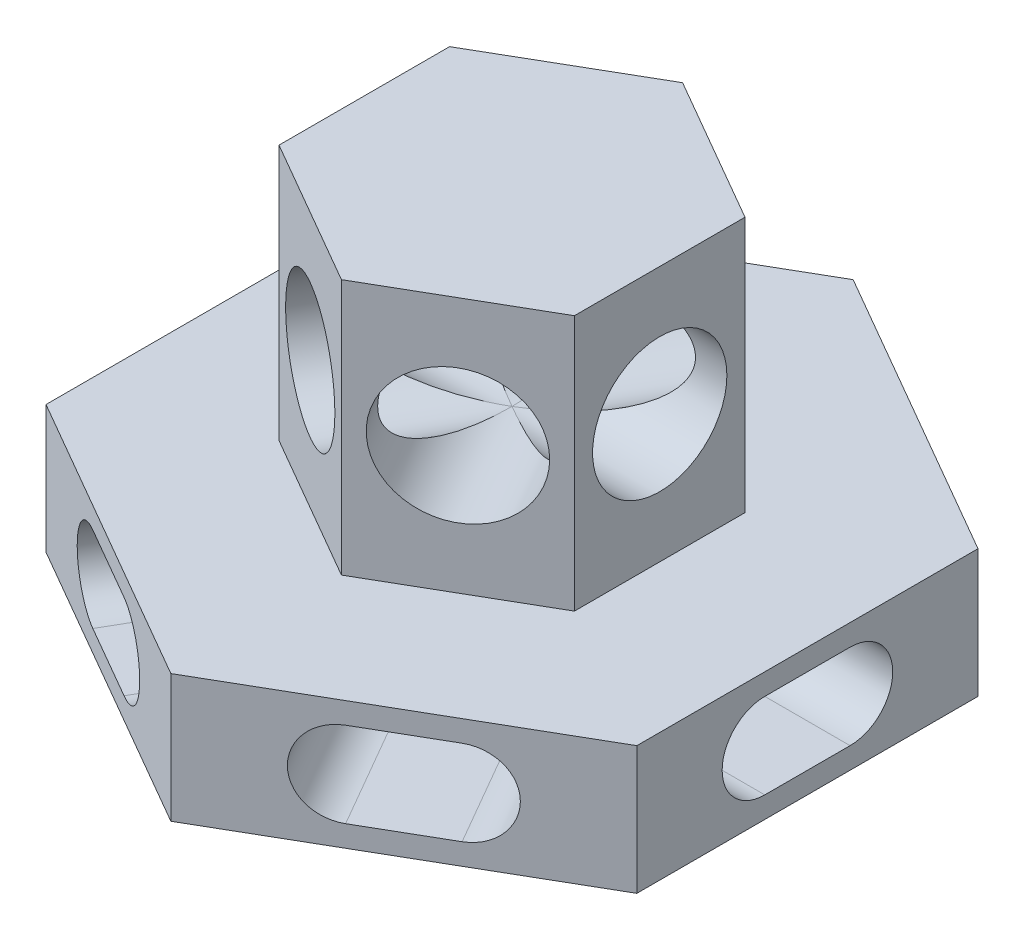
ISO-10303-21;
HEADER;
FILE_DESCRIPTION(('STEP AP214'),'2;1');
FILE_NAME('part.step','',(''),(''),'','','');
FILE_SCHEMA(('AUTOMOTIVE_DESIGN { 1 0 10303 214 1 1 1 1 }'));
ENDSEC;
DATA;
#1=APPLICATION_CONTEXT('core data for automotive mechanical design processes');
#2=APPLICATION_PROTOCOL_DEFINITION('international standard','automotive_design',2000,#1);
#3=PRODUCT_CONTEXT('',#1,'mechanical');
#4=PRODUCT('Part','Part','',(#3));
#5=PRODUCT_RELATED_PRODUCT_CATEGORY('part','',(#4));
#6=PRODUCT_DEFINITION_FORMATION('','',#4);
#7=PRODUCT_DEFINITION_CONTEXT('part definition',#1,'design');
#8=PRODUCT_DEFINITION('design','',#6,#7);
#9=PRODUCT_DEFINITION_SHAPE('','',#8);
#10=(LENGTH_UNIT() NAMED_UNIT(*) SI_UNIT(.MILLI.,.METRE.));
#11=(NAMED_UNIT(*) PLANE_ANGLE_UNIT() SI_UNIT($,.RADIAN.));
#12=(NAMED_UNIT(*) SI_UNIT($,.STERADIAN.) SOLID_ANGLE_UNIT());
#13=UNCERTAINTY_MEASURE_WITH_UNIT(LENGTH_MEASURE(1.E-05),#10,'distance_accuracy_value','');
#14=(GEOMETRIC_REPRESENTATION_CONTEXT(3) GLOBAL_UNCERTAINTY_ASSIGNED_CONTEXT((#13)) GLOBAL_UNIT_ASSIGNED_CONTEXT((#10,
#11,#12)) REPRESENTATION_CONTEXT('',''));
#15=CARTESIAN_POINT('',(0.,0.,0.));
#16=DIRECTION('',(0.,0.,1.));
#17=DIRECTION('',(1.,0.,0.));
#18=AXIS2_PLACEMENT_3D('',#15,#16,#17);
#19=CARTESIAN_POINT('',(-69.2820323027551,45.,0.));
#20=DIRECTION('',(1.,0.,0.));
#21=DIRECTION('',(0.,0.,-1.));
#22=AXIS2_PLACEMENT_3D('',#19,#20,#21);
#23=CYLINDRICAL_SURFACE('',#22,15.75);
#24=CARTESIAN_POINT('',(34.6410161513775,45.,0.));
#25=DIRECTION('',(1.,0.,0.));
#26=DIRECTION('',(0.,0.,-1.));
#27=AXIS2_PLACEMENT_3D('',#24,#25,#26);
#28=CIRCLE('',#27,15.75);
#29=CARTESIAN_POINT('',(34.6410161513775,45.,-15.75));
#30=VERTEX_POINT('',#29);
#31=EDGE_CURVE('E278',#30,#30,#28,.T.);
#32=ORIENTED_EDGE('',*,*,#31,.T.);
#33=EDGE_LOOP('',(#32));
#34=FACE_BOUND('',#33,.T.);
#35=CARTESIAN_POINT('',(0.,45.,0.));
#36=DIRECTION('',(0.5,0.,0.866025403784439));
#37=DIRECTION('',(0.866025403784439,0.,-0.5));
#38=AXIS2_PLACEMENT_3D('',#35,#36,#37);
#39=ELLIPSE('',#38,31.5,15.75);
#40=CARTESIAN_POINT('',(0.,60.75,0.));
#41=VERTEX_POINT('',#40);
#42=CARTESIAN_POINT('',(0.,29.25,0.));
#43=VERTEX_POINT('',#42);
#44=EDGE_CURVE('E262',#41,#43,#39,.F.);
#45=ORIENTED_EDGE('',*,*,#44,.T.);
#46=CARTESIAN_POINT('',(0.,45.,0.));
#47=DIRECTION('',(0.5,0.,-0.866025403784439));
#48=DIRECTION('',(0.866025403784439,0.,0.5));
#49=AXIS2_PLACEMENT_3D('',#46,#47,#48);
#50=ELLIPSE('',#49,31.5,15.75);
#51=EDGE_CURVE('E260',#43,#41,#50,.F.);
#52=ORIENTED_EDGE('',*,*,#51,.T.);
#53=EDGE_LOOP('',(#45,#52));
#54=FACE_BOUND('',#53,.T.);
#55=ADVANCED_FACE('F41',(#34,#54),#23,.F.);
#56=CARTESIAN_POINT('',(69.2820323027551,0.,-9.99999999999999));
#57=DIRECTION('',(-1.,0.,0.));
#58=DIRECTION('',(0.,0.,1.));
#59=AXIS2_PLACEMENT_3D('',#56,#57,#58);
#60=CYLINDRICAL_SURFACE('',#59,10.);
#61=DIRECTION('',(-1.,0.,0.));
#62=VECTOR('',#61,1.);
#63=CARTESIAN_POINT('',(69.2820323027551,10.,-9.99999999999999));
#64=LINE('',#63,#62);
#65=CARTESIAN_POINT('',(69.2820323027551,10.,-9.99999999999999));
#66=VERTEX_POINT('',#65);
#67=CARTESIAN_POINT('',(17.3205080756888,10.,-9.99999999999998));
#68=VERTEX_POINT('',#67);
#69=EDGE_CURVE('E438',#66,#68,#64,.T.);
#70=ORIENTED_EDGE('',*,*,#69,.T.);
#71=CARTESIAN_POINT('',(17.3205080756888,0.,-9.99999999999999));
#72=DIRECTION('',(-0.5,0.,-0.866025403784439));
#73=DIRECTION('',(-0.866025403784439,0.,0.5));
#74=AXIS2_PLACEMENT_3D('',#71,#72,#73);
#75=ELLIPSE('',#74,20.,10.);
#76=CARTESIAN_POINT('',(17.3205080756888,-10.,-9.99999999999998));
#77=VERTEX_POINT('',#76);
#78=EDGE_CURVE('E405',#68,#77,#75,.T.);
#79=ORIENTED_EDGE('',*,*,#78,.T.);
#80=DIRECTION('',(-1.,0.,0.));
#81=VECTOR('',#80,1.);
#82=CARTESIAN_POINT('',(69.2820323027551,-10.,-9.99999999999999));
#83=LINE('',#82,#81);
#84=CARTESIAN_POINT('',(69.2820323027551,-10.,-9.99999999999999));
#85=VERTEX_POINT('',#84);
#86=EDGE_CURVE('E455',#85,#77,#83,.T.);
#87=ORIENTED_EDGE('',*,*,#86,.F.);
#88=CARTESIAN_POINT('',(69.2820323027551,0.,-9.99999999999999));
#89=DIRECTION('',(-1.,0.,0.));
#90=DIRECTION('',(0.,0.,1.));
#91=AXIS2_PLACEMENT_3D('',#88,#89,#90);
#92=CIRCLE('',#91,10.);
#93=EDGE_CURVE('E414',#66,#85,#92,.T.);
#94=ORIENTED_EDGE('',*,*,#93,.F.);
#95=EDGE_LOOP('',(#70,#79,#87,#94));
#96=FACE_BOUND('',#95,.T.);
#97=ADVANCED_FACE('F525',(#96),#60,.F.);
#98=CARTESIAN_POINT('',(69.2820323027551,0.,10.));
#99=DIRECTION('',(-1.,0.,0.));
#100=DIRECTION('',(0.,0.,1.));
#101=AXIS2_PLACEMENT_3D('',#98,#99,#100);
#102=CYLINDRICAL_SURFACE('',#101,10.);
#103=DIRECTION('',(-1.,0.,0.));
#104=VECTOR('',#103,1.);
#105=CARTESIAN_POINT('',(69.2820323027551,-10.,10.));
#106=LINE('',#105,#104);
#107=CARTESIAN_POINT('',(69.2820323027551,-10.,10.));
#108=VERTEX_POINT('',#107);
#109=CARTESIAN_POINT('',(17.3205080756888,-10.,9.99999999999999));
#110=VERTEX_POINT('',#109);
#111=EDGE_CURVE('E450',#108,#110,#106,.T.);
#112=ORIENTED_EDGE('',*,*,#111,.T.);
#113=CARTESIAN_POINT('',(17.3205080756888,0.,10.));
#114=DIRECTION('',(-0.5,0.,0.866025403784439));
#115=DIRECTION('',(-0.866025403784439,0.,-0.5));
#116=AXIS2_PLACEMENT_3D('',#113,#114,#115);
#117=ELLIPSE('',#116,20.,10.);
#118=CARTESIAN_POINT('',(17.3205080756888,10.,9.99999999999999));
#119=VERTEX_POINT('',#118);
#120=EDGE_CURVE('E361',#110,#119,#117,.T.);
#121=ORIENTED_EDGE('',*,*,#120,.T.);
#122=DIRECTION('',(-1.,0.,0.));
#123=VECTOR('',#122,1.);
#124=CARTESIAN_POINT('',(69.2820323027551,10.,10.));
#125=LINE('',#124,#123);
#126=CARTESIAN_POINT('',(69.2820323027551,10.,10.));
#127=VERTEX_POINT('',#126);
#128=EDGE_CURVE('E441',#127,#119,#125,.T.);
#129=ORIENTED_EDGE('',*,*,#128,.F.);
#130=CARTESIAN_POINT('',(69.2820323027551,0.,10.));
#131=DIRECTION('',(-1.,0.,0.));
#132=DIRECTION('',(0.,0.,1.));
#133=AXIS2_PLACEMENT_3D('',#130,#131,#132);
#134=CIRCLE('',#133,10.);
#135=EDGE_CURVE('E425',#108,#127,#134,.T.);
#136=ORIENTED_EDGE('',*,*,#135,.F.);
#137=EDGE_LOOP('',(#112,#121,#129,#136));
#138=FACE_BOUND('',#137,.T.);
#139=ADVANCED_FACE('F530',(#138),#102,.F.);
#140=CARTESIAN_POINT('',(0.,15.,80.));
#141=DIRECTION('',(-0.499999999999999,0.,-0.866025403784439));
#142=DIRECTION('',(-0.866025403784439,0.,0.5));
#143=AXIS2_PLACEMENT_3D('',#140,#141,#142);
#144=PLANE('',#143);
#145=DIRECTION('',(0.866025403784439,0.,-0.5));
#146=VECTOR('',#145,1.);
#147=CARTESIAN_POINT('',(0.,10.,80.));
#148=LINE('',#147,#146);
#149=CARTESIAN_POINT('',(25.9807621135331,10.,65.));
#150=VERTEX_POINT('',#149);
#151=CARTESIAN_POINT('',(43.3012701892219,10.,55.));
#152=VERTEX_POINT('',#151);
#153=EDGE_CURVE('E360',#150,#152,#148,.T.);
#154=ORIENTED_EDGE('',*,*,#153,.T.);
#155=CARTESIAN_POINT('',(43.3012701892219,0.,55.));
#156=DIRECTION('',(-0.499999999999999,0.,-0.866025403784439));
#157=DIRECTION('',(-0.866025403784439,0.,0.5));
#158=AXIS2_PLACEMENT_3D('',#155,#156,#157);
#159=CIRCLE('',#158,10.);
#160=CARTESIAN_POINT('',(43.3012701892219,-10.,55.));
#161=VERTEX_POINT('',#160);
#162=EDGE_CURVE('E359',#152,#161,#159,.T.);
#163=ORIENTED_EDGE('',*,*,#162,.T.);
#164=DIRECTION('',(-0.866025403784439,0.,0.5));
#165=VECTOR('',#164,1.);
#166=CARTESIAN_POINT('',(0.,-9.99999999999999,80.));
#167=LINE('',#166,#165);
#168=CARTESIAN_POINT('',(25.9807621135331,-10.,65.));
#169=VERTEX_POINT('',#168);
#170=EDGE_CURVE('E351',#161,#169,#167,.T.);
#171=ORIENTED_EDGE('',*,*,#170,.T.);
#172=CARTESIAN_POINT('',(25.9807621135331,0.,65.));
#173=DIRECTION('',(-0.499999999999999,0.,-0.866025403784439));
#174=DIRECTION('',(-0.866025403784439,0.,0.5));
#175=AXIS2_PLACEMENT_3D('',#172,#173,#174);
#176=CIRCLE('',#175,10.);
#177=EDGE_CURVE('E369',#169,#150,#176,.T.);
#178=ORIENTED_EDGE('',*,*,#177,.T.);
#179=EDGE_LOOP('',(#154,#163,#171,#178));
#180=FACE_BOUND('',#179,.T.);
#181=DIRECTION('',(0.866025403784439,0.,-0.5));
#182=VECTOR('',#181,1.);
#183=CARTESIAN_POINT('',(0.,-15.,80.));
#184=LINE('',#183,#182);
#185=CARTESIAN_POINT('',(0.,-15.,80.));
#186=VERTEX_POINT('',#185);
#187=CARTESIAN_POINT('',(69.2820323027551,-15.,40.));
#188=VERTEX_POINT('',#187);
#189=EDGE_CURVE('E445',#186,#188,#184,.T.);
#190=ORIENTED_EDGE('',*,*,#189,.T.);
#191=DIRECTION('',(0.,-1.,0.));
#192=VECTOR('',#191,1.);
#193=CARTESIAN_POINT('',(69.2820323027551,15.,40.));
#194=LINE('',#193,#192);
#195=CARTESIAN_POINT('',(69.2820323027551,15.,40.));
#196=VERTEX_POINT('',#195);
#197=EDGE_CURVE('E494',#196,#188,#194,.T.);
#198=ORIENTED_EDGE('',*,*,#197,.F.);
#199=DIRECTION('',(0.866025403784439,0.,-0.5));
#200=VECTOR('',#199,1.);
#201=CARTESIAN_POINT('',(0.,15.,80.));
#202=LINE('',#201,#200);
#203=CARTESIAN_POINT('',(0.,15.,80.));
#204=VERTEX_POINT('',#203);
#205=EDGE_CURVE('E454',#204,#196,#202,.T.);
#206=ORIENTED_EDGE('',*,*,#205,.F.);
#207=DIRECTION('',(0.,-1.,0.));
#208=VECTOR('',#207,1.);
#209=CARTESIAN_POINT('',(0.,15.,80.));
#210=LINE('',#209,#208);
#211=EDGE_CURVE('E467',#204,#186,#210,.T.);
#212=ORIENTED_EDGE('',*,*,#211,.T.);
#213=EDGE_LOOP('',(#190,#198,#206,#212));
#214=FACE_BOUND('',#213,.T.);
#215=ADVANCED_FACE('F43',(#180,#214),#144,.F.);
#216=CARTESIAN_POINT('',(69.2820323027551,15.,40.));
#217=DIRECTION('',(-1.,0.,0.));
#218=DIRECTION('',(0.,0.,1.));
#219=AXIS2_PLACEMENT_3D('',#216,#217,#218);
#220=PLANE('',#219);
#221=DIRECTION('',(0.,0.,-1.));
#222=VECTOR('',#221,1.);
#223=CARTESIAN_POINT('',(69.2820323027551,10.,-9.99999999999999));
#224=LINE('',#223,#222);
#225=EDGE_CURVE('E422',#127,#66,#224,.T.);
#226=ORIENTED_EDGE('',*,*,#225,.T.);
#227=ORIENTED_EDGE('',*,*,#93,.T.);
#228=DIRECTION('',(0.,0.,1.));
#229=VECTOR('',#228,1.);
#230=CARTESIAN_POINT('',(69.2820323027551,-10.,-9.99999999999999));
#231=LINE('',#230,#229);
#232=EDGE_CURVE('E416',#85,#108,#231,.T.);
#233=ORIENTED_EDGE('',*,*,#232,.T.);
#234=ORIENTED_EDGE('',*,*,#135,.T.);
#235=EDGE_LOOP('',(#226,#227,#233,#234));
#236=FACE_BOUND('',#235,.T.);
#237=DIRECTION('',(0.,0.,-1.));
#238=VECTOR('',#237,1.);
#239=CARTESIAN_POINT('',(69.2820323027551,-15.,40.));
#240=LINE('',#239,#238);
#241=CARTESIAN_POINT('',(69.2820323027551,-15.,-40.));
#242=VERTEX_POINT('',#241);
#243=EDGE_CURVE('E472',#188,#242,#240,.T.);
#244=ORIENTED_EDGE('',*,*,#243,.T.);
#245=DIRECTION('',(0.,-1.,0.));
#246=VECTOR('',#245,1.);
#247=CARTESIAN_POINT('',(69.2820323027551,15.,-40.));
#248=LINE('',#247,#246);
#249=CARTESIAN_POINT('',(69.2820323027551,15.,-40.));
#250=VERTEX_POINT('',#249);
#251=EDGE_CURVE('E495',#250,#242,#248,.T.);
#252=ORIENTED_EDGE('',*,*,#251,.F.);
#253=DIRECTION('',(0.,0.,-1.));
#254=VECTOR('',#253,1.);
#255=CARTESIAN_POINT('',(69.2820323027551,15.,40.));
#256=LINE('',#255,#254);
#257=EDGE_CURVE('E456',#196,#250,#256,.T.);
#258=ORIENTED_EDGE('',*,*,#257,.F.);
#259=ORIENTED_EDGE('',*,*,#197,.T.);
#260=EDGE_LOOP('',(#244,#252,#258,#259));
#261=FACE_BOUND('',#260,.T.);
#262=ADVANCED_FACE('F627',(#236,#261),#220,.F.);
#263=CARTESIAN_POINT('',(69.2820323027551,15.,-40.));
#264=DIRECTION('',(-0.5,0.,0.866025403784439));
#265=DIRECTION('',(0.866025403784439,0.,0.5));
#266=AXIS2_PLACEMENT_3D('',#263,#264,#265);
#267=PLANE('',#266);
#268=DIRECTION('',(-0.866025403784438,0.,-0.5));
#269=VECTOR('',#268,1.);
#270=CARTESIAN_POINT('',(43.301270189222,-10.,-55.));
#271=LINE('',#270,#269);
#272=CARTESIAN_POINT('',(43.301270189222,-10.,-55.));
#273=VERTEX_POINT('',#272);
#274=CARTESIAN_POINT('',(25.9807621135332,-10.,-65.));
#275=VERTEX_POINT('',#274);
#276=EDGE_CURVE('E372',#273,#275,#271,.T.);
#277=ORIENTED_EDGE('',*,*,#276,.F.);
#278=CARTESIAN_POINT('',(43.301270189222,0.,-55.));
#279=DIRECTION('',(0.5,0.,-0.866025403784438));
#280=DIRECTION('',(-0.866025403784439,0.,-0.5));
#281=AXIS2_PLACEMENT_3D('',#278,#279,#280);
#282=CIRCLE('',#281,10.);
#283=CARTESIAN_POINT('',(43.301270189222,10.,-55.));
#284=VERTEX_POINT('',#283);
#285=EDGE_CURVE('E375',#284,#273,#282,.T.);
#286=ORIENTED_EDGE('',*,*,#285,.F.);
#287=DIRECTION('',(0.866025403784438,0.,0.5));
#288=VECTOR('',#287,1.);
#289=CARTESIAN_POINT('',(43.301270189222,10.,-55.));
#290=LINE('',#289,#288);
#291=CARTESIAN_POINT('',(25.9807621135332,10.,-65.));
#292=VERTEX_POINT('',#291);
#293=EDGE_CURVE('E379',#292,#284,#290,.T.);
#294=ORIENTED_EDGE('',*,*,#293,.F.);
#295=CARTESIAN_POINT('',(25.9807621135332,0.,-65.));
#296=DIRECTION('',(0.5,0.,-0.866025403784438));
#297=DIRECTION('',(-0.866025403784439,0.,-0.5));
#298=AXIS2_PLACEMENT_3D('',#295,#296,#297);
#299=CIRCLE('',#298,10.);
#300=EDGE_CURVE('E380',#275,#292,#299,.T.);
#301=ORIENTED_EDGE('',*,*,#300,.F.);
#302=EDGE_LOOP('',(#277,#286,#294,#301));
#303=FACE_BOUND('',#302,.T.);
#304=DIRECTION('',(-0.866025403784439,0.,-0.5));
#305=VECTOR('',#304,1.);
#306=CARTESIAN_POINT('',(69.2820323027551,-15.,-40.));
#307=LINE('',#306,#305);
#308=CARTESIAN_POINT('',(0.,-15.,-80.));
#309=VERTEX_POINT('',#308);
#310=EDGE_CURVE('E475',#242,#309,#307,.T.);
#311=ORIENTED_EDGE('',*,*,#310,.T.);
#312=DIRECTION('',(0.,-1.,0.));
#313=VECTOR('',#312,1.);
#314=CARTESIAN_POINT('',(0.,15.,-80.));
#315=LINE('',#314,#313);
#316=CARTESIAN_POINT('',(0.,15.,-80.));
#317=VERTEX_POINT('',#316);
#318=EDGE_CURVE('E487',#317,#309,#315,.T.);
#319=ORIENTED_EDGE('',*,*,#318,.F.);
#320=DIRECTION('',(-0.866025403784439,0.,-0.5));
#321=VECTOR('',#320,1.);
#322=CARTESIAN_POINT('',(69.2820323027551,15.,-40.));
#323=LINE('',#322,#321);
#324=EDGE_CURVE('E462',#250,#317,#323,.T.);
#325=ORIENTED_EDGE('',*,*,#324,.F.);
#326=ORIENTED_EDGE('',*,*,#251,.T.);
#327=EDGE_LOOP('',(#311,#319,#325,#326));
#328=FACE_BOUND('',#327,.T.);
#329=ADVANCED_FACE('F621',(#303,#328),#267,.F.);
#330=CARTESIAN_POINT('',(0.,15.,-80.));
#331=DIRECTION('',(0.5,0.,0.866025403784439));
#332=DIRECTION('',(0.866025403784439,0.,-0.5));
#333=AXIS2_PLACEMENT_3D('',#330,#331,#332);
#334=PLANE('',#333);
#335=DIRECTION('',(-0.866025403784439,0.,0.5));
#336=VECTOR('',#335,1.);
#337=CARTESIAN_POINT('',(-25.9807621135332,-10.,-65.));
#338=LINE('',#337,#336);
#339=CARTESIAN_POINT('',(-25.9807621135331,-10.,-65.));
#340=VERTEX_POINT('',#339);
#341=CARTESIAN_POINT('',(-43.3012701892219,-10.,-55.));
#342=VERTEX_POINT('',#341);
#343=EDGE_CURVE('E335',#340,#342,#338,.T.);
#344=ORIENTED_EDGE('',*,*,#343,.F.);
#345=CARTESIAN_POINT('',(-25.9807621135332,0.,-65.));
#346=DIRECTION('',(-0.5,0.,-0.866025403784439));
#347=DIRECTION('',(-0.866025403784439,0.,0.5));
#348=AXIS2_PLACEMENT_3D('',#345,#346,#347);
#349=CIRCLE('',#348,10.);
#350=CARTESIAN_POINT('',(-25.9807621135332,10.,-65.));
#351=VERTEX_POINT('',#350);
#352=EDGE_CURVE('E329',#351,#340,#349,.T.);
#353=ORIENTED_EDGE('',*,*,#352,.F.);
#354=DIRECTION('',(0.866025403784439,0.,-0.5));
#355=VECTOR('',#354,1.);
#356=CARTESIAN_POINT('',(-25.9807621135332,10.,-65.));
#357=LINE('',#356,#355);
#358=CARTESIAN_POINT('',(-43.3012701892219,10.,-55.));
#359=VERTEX_POINT('',#358);
#360=EDGE_CURVE('E340',#359,#351,#357,.T.);
#361=ORIENTED_EDGE('',*,*,#360,.F.);
#362=CARTESIAN_POINT('',(-43.3012701892219,0.,-55.));
#363=DIRECTION('',(-0.5,0.,-0.866025403784439));
#364=DIRECTION('',(-0.866025403784439,0.,0.5));
#365=AXIS2_PLACEMENT_3D('',#362,#363,#364);
#366=CIRCLE('',#365,10.);
#367=EDGE_CURVE('E333',#342,#359,#366,.T.);
#368=ORIENTED_EDGE('',*,*,#367,.F.);
#369=EDGE_LOOP('',(#344,#353,#361,#368));
#370=FACE_BOUND('',#369,.T.);
#371=DIRECTION('',(-0.866025403784439,0.,0.5));
#372=VECTOR('',#371,1.);
#373=CARTESIAN_POINT('',(0.,-15.,-80.));
#374=LINE('',#373,#372);
#375=CARTESIAN_POINT('',(-69.2820323027551,-15.,-40.));
#376=VERTEX_POINT('',#375);
#377=EDGE_CURVE('E478',#309,#376,#374,.T.);
#378=ORIENTED_EDGE('',*,*,#377,.T.);
#379=DIRECTION('',(0.,-1.,0.));
#380=VECTOR('',#379,1.);
#381=CARTESIAN_POINT('',(-69.2820323027551,15.,-40.));
#382=LINE('',#381,#380);
#383=CARTESIAN_POINT('',(-69.2820323027551,15.,-40.));
#384=VERTEX_POINT('',#383);
#385=EDGE_CURVE('E486',#384,#376,#382,.T.);
#386=ORIENTED_EDGE('',*,*,#385,.F.);
#387=DIRECTION('',(-0.866025403784439,0.,0.5));
#388=VECTOR('',#387,1.);
#389=CARTESIAN_POINT('',(0.,15.,-80.));
#390=LINE('',#389,#388);
#391=EDGE_CURVE('E465',#317,#384,#390,.T.);
#392=ORIENTED_EDGE('',*,*,#391,.F.);
#393=ORIENTED_EDGE('',*,*,#318,.T.);
#394=EDGE_LOOP('',(#378,#386,#392,#393));
#395=FACE_BOUND('',#394,.T.);
#396=ADVANCED_FACE('F617',(#370,#395),#334,.F.);
#397=CARTESIAN_POINT('',(-69.2820323027551,15.,-40.));
#398=DIRECTION('',(1.,0.,0.));
#399=DIRECTION('',(0.,0.,-1.));
#400=AXIS2_PLACEMENT_3D('',#397,#398,#399);
#401=PLANE('',#400);
#402=DIRECTION('',(0.,0.,1.));
#403=VECTOR('',#402,1.);
#404=CARTESIAN_POINT('',(-69.2820323027551,-10.,-10.));
#405=LINE('',#404,#403);
#406=CARTESIAN_POINT('',(-69.2820323027551,-10.,-10.));
#407=VERTEX_POINT('',#406);
#408=CARTESIAN_POINT('',(-69.2820323027551,-10.,9.99999999999999));
#409=VERTEX_POINT('',#408);
#410=EDGE_CURVE('E431',#407,#409,#405,.T.);
#411=ORIENTED_EDGE('',*,*,#410,.F.);
#412=CARTESIAN_POINT('',(-69.2820323027551,0.,-10.));
#413=DIRECTION('',(-1.,0.,0.));
#414=DIRECTION('',(0.,0.,1.));
#415=AXIS2_PLACEMENT_3D('',#412,#413,#414);
#416=CIRCLE('',#415,10.);
#417=CARTESIAN_POINT('',(-69.2820323027551,10.,-10.));
#418=VERTEX_POINT('',#417);
#419=EDGE_CURVE('E412',#418,#407,#416,.T.);
#420=ORIENTED_EDGE('',*,*,#419,.F.);
#421=DIRECTION('',(0.,0.,-1.));
#422=VECTOR('',#421,1.);
#423=CARTESIAN_POINT('',(-69.2820323027551,10.,-10.));
#424=LINE('',#423,#422);
#425=CARTESIAN_POINT('',(-69.2820323027551,10.,9.99999999999998));
#426=VERTEX_POINT('',#425);
#427=EDGE_CURVE('E420',#426,#418,#424,.T.);
#428=ORIENTED_EDGE('',*,*,#427,.F.);
#429=CARTESIAN_POINT('',(-69.2820323027551,0.,9.99999999999999));
#430=DIRECTION('',(-1.,0.,0.));
#431=DIRECTION('',(0.,0.,1.));
#432=AXIS2_PLACEMENT_3D('',#429,#430,#431);
#433=CIRCLE('',#432,10.);
#434=EDGE_CURVE('E432',#409,#426,#433,.T.);
#435=ORIENTED_EDGE('',*,*,#434,.F.);
#436=EDGE_LOOP('',(#411,#420,#428,#435));
#437=FACE_BOUND('',#436,.T.);
#438=DIRECTION('',(0.,0.,1.));
#439=VECTOR('',#438,1.);
#440=CARTESIAN_POINT('',(-69.2820323027551,-15.,-40.));
#441=LINE('',#440,#439);
#442=CARTESIAN_POINT('',(-69.2820323027551,-15.,40.));
#443=VERTEX_POINT('',#442);
#444=EDGE_CURVE('E476',#376,#443,#441,.T.);
#445=ORIENTED_EDGE('',*,*,#444,.T.);
#446=DIRECTION('',(0.,-1.,0.));
#447=VECTOR('',#446,1.);
#448=CARTESIAN_POINT('',(-69.2820323027551,15.,40.));
#449=LINE('',#448,#447);
#450=CARTESIAN_POINT('',(-69.2820323027551,15.,40.));
#451=VERTEX_POINT('',#450);
#452=EDGE_CURVE('E483',#451,#443,#449,.T.);
#453=ORIENTED_EDGE('',*,*,#452,.F.);
#454=DIRECTION('',(0.,0.,1.));
#455=VECTOR('',#454,1.);
#456=CARTESIAN_POINT('',(-69.2820323027551,15.,-40.));
#457=LINE('',#456,#455);
#458=EDGE_CURVE('E463',#384,#451,#457,.T.);
#459=ORIENTED_EDGE('',*,*,#458,.F.);
#460=ORIENTED_EDGE('',*,*,#385,.T.);
#461=EDGE_LOOP('',(#445,#453,#459,#460));
#462=FACE_BOUND('',#461,.T.);
#463=ADVANCED_FACE('F613',(#437,#462),#401,.F.);
#464=CARTESIAN_POINT('',(-69.2820323027551,15.,40.));
#465=DIRECTION('',(0.5,0.,-0.866025403784439));
#466=DIRECTION('',(-0.866025403784439,0.,-0.5));
#467=AXIS2_PLACEMENT_3D('',#464,#465,#466);
#468=PLANE('',#467);
#469=DIRECTION('',(0.866025403784439,0.,0.5));
#470=VECTOR('',#469,1.);
#471=CARTESIAN_POINT('',(-69.2820323027551,10.,40.));
#472=LINE('',#471,#470);
#473=CARTESIAN_POINT('',(-43.3012701892219,10.,55.));
#474=VERTEX_POINT('',#473);
#475=CARTESIAN_POINT('',(-25.9807621135332,10.,65.));
#476=VERTEX_POINT('',#475);
#477=EDGE_CURVE('E413',#474,#476,#472,.T.);
#478=ORIENTED_EDGE('',*,*,#477,.T.);
#479=CARTESIAN_POINT('',(-25.9807621135332,0.,65.));
#480=DIRECTION('',(0.5,0.,-0.866025403784439));
#481=DIRECTION('',(-0.866025403784439,0.,-0.5));
#482=AXIS2_PLACEMENT_3D('',#479,#480,#481);
#483=CIRCLE('',#482,10.);
#484=CARTESIAN_POINT('',(-25.9807621135332,-10.,65.));
#485=VERTEX_POINT('',#484);
#486=EDGE_CURVE('E403',#476,#485,#483,.T.);
#487=ORIENTED_EDGE('',*,*,#486,.T.);
#488=DIRECTION('',(-0.866025403784439,0.,-0.5));
#489=VECTOR('',#488,1.);
#490=CARTESIAN_POINT('',(-69.2820323027551,-9.99999999999999,40.));
#491=LINE('',#490,#489);
#492=CARTESIAN_POINT('',(-43.301270189222,-10.,55.));
#493=VERTEX_POINT('',#492);
#494=EDGE_CURVE('E410',#485,#493,#491,.T.);
#495=ORIENTED_EDGE('',*,*,#494,.T.);
#496=CARTESIAN_POINT('',(-43.301270189222,0.,55.));
#497=DIRECTION('',(0.5,0.,-0.866025403784439));
#498=DIRECTION('',(-0.866025403784439,0.,-0.5));
#499=AXIS2_PLACEMENT_3D('',#496,#497,#498);
#500=CIRCLE('',#499,10.);
#501=EDGE_CURVE('E397',#493,#474,#500,.T.);
#502=ORIENTED_EDGE('',*,*,#501,.T.);
#503=EDGE_LOOP('',(#478,#487,#495,#502));
#504=FACE_BOUND('',#503,.T.);
#505=DIRECTION('',(0.866025403784439,0.,0.5));
#506=VECTOR('',#505,1.);
#507=CARTESIAN_POINT('',(-69.2820323027551,-15.,40.));
#508=LINE('',#507,#506);
#509=EDGE_CURVE('E459',#443,#186,#508,.T.);
#510=ORIENTED_EDGE('',*,*,#509,.T.);
#511=ORIENTED_EDGE('',*,*,#211,.F.);
#512=DIRECTION('',(0.866025403784439,0.,0.5));
#513=VECTOR('',#512,1.);
#514=CARTESIAN_POINT('',(-69.2820323027551,15.,40.));
#515=LINE('',#514,#513);
#516=EDGE_CURVE('E470',#451,#204,#515,.T.);
#517=ORIENTED_EDGE('',*,*,#516,.F.);
#518=ORIENTED_EDGE('',*,*,#452,.T.);
#519=EDGE_LOOP('',(#510,#511,#517,#518));
#520=FACE_BOUND('',#519,.T.);
#521=ADVANCED_FACE('F606',(#504,#520),#468,.F.);
#522=CARTESIAN_POINT('',(0.,15.,0.));
#523=DIRECTION('',(0.,1.,0.));
#524=DIRECTION('',(0.,0.,1.));
#525=AXIS2_PLACEMENT_3D('',#522,#523,#524);
#526=PLANE('',#525);
#527=DIRECTION('',(0.866025403784439,0.,-0.5));
#528=VECTOR('',#527,1.);
#529=CARTESIAN_POINT('',(0.,15.,40.));
#530=LINE('',#529,#528);
#531=CARTESIAN_POINT('',(0.,15.,40.));
#532=VERTEX_POINT('',#531);
#533=CARTESIAN_POINT('',(34.6410161513775,15.,20.));
#534=VERTEX_POINT('',#533);
#535=EDGE_CURVE('E62',#532,#534,#530,.T.);
#536=ORIENTED_EDGE('',*,*,#535,.F.);
#537=DIRECTION('',(0.866025403784438,0.,0.5));
#538=VECTOR('',#537,1.);
#539=CARTESIAN_POINT('',(-34.6410161513776,15.,20.));
#540=LINE('',#539,#538);
#541=CARTESIAN_POINT('',(-34.6410161513776,15.,20.));
#542=VERTEX_POINT('',#541);
#543=EDGE_CURVE('E286',#542,#532,#540,.T.);
#544=ORIENTED_EDGE('',*,*,#543,.F.);
#545=DIRECTION('',(0.,0.,1.));
#546=VECTOR('',#545,1.);
#547=CARTESIAN_POINT('',(-34.6410161513775,15.,-20.));
#548=LINE('',#547,#546);
#549=CARTESIAN_POINT('',(-34.6410161513775,15.,-20.));
#550=VERTEX_POINT('',#549);
#551=EDGE_CURVE('E310',#550,#542,#548,.T.);
#552=ORIENTED_EDGE('',*,*,#551,.F.);
#553=DIRECTION('',(-0.866025403784439,0.,0.499999999999999));
#554=VECTOR('',#553,1.);
#555=CARTESIAN_POINT('',(0.,15.,-40.));
#556=LINE('',#555,#554);
#557=CARTESIAN_POINT('',(0.,15.,-40.));
#558=VERTEX_POINT('',#557);
#559=EDGE_CURVE('E308',#558,#550,#556,.T.);
#560=ORIENTED_EDGE('',*,*,#559,.F.);
#561=DIRECTION('',(-0.866025403784438,0.,-0.5));
#562=VECTOR('',#561,1.);
#563=CARTESIAN_POINT('',(34.6410161513775,15.,-20.));
#564=LINE('',#563,#562);
#565=CARTESIAN_POINT('',(34.6410161513775,15.,-20.));
#566=VERTEX_POINT('',#565);
#567=EDGE_CURVE('E301',#566,#558,#564,.T.);
#568=ORIENTED_EDGE('',*,*,#567,.F.);
#569=DIRECTION('',(0.,0.,-1.));
#570=VECTOR('',#569,1.);
#571=CARTESIAN_POINT('',(34.6410161513775,15.,20.));
#572=LINE('',#571,#570);
#573=EDGE_CURVE('E298',#534,#566,#572,.T.);
#574=ORIENTED_EDGE('',*,*,#573,.F.);
#575=EDGE_LOOP('',(#536,#544,#552,#560,#568,#574));
#576=FACE_BOUND('',#575,.T.);
#577=ORIENTED_EDGE('',*,*,#205,.T.);
#578=ORIENTED_EDGE('',*,*,#257,.T.);
#579=ORIENTED_EDGE('',*,*,#324,.T.);
#580=ORIENTED_EDGE('',*,*,#391,.T.);
#581=ORIENTED_EDGE('',*,*,#458,.T.);
#582=ORIENTED_EDGE('',*,*,#516,.T.);
#583=EDGE_LOOP('',(#577,#578,#579,#580,#581,#582));
#584=FACE_BOUND('',#583,.T.);
#585=ADVANCED_FACE('F551',(#576,#584),#526,.T.);
#586=CARTESIAN_POINT('',(0.,-15.,0.));
#587=DIRECTION('',(0.,1.,0.));
#588=DIRECTION('',(0.,0.,1.));
#589=AXIS2_PLACEMENT_3D('',#586,#587,#588);
#590=PLANE('',#589);
#591=ORIENTED_EDGE('',*,*,#189,.F.);
#592=ORIENTED_EDGE('',*,*,#509,.F.);
#593=ORIENTED_EDGE('',*,*,#444,.F.);
#594=ORIENTED_EDGE('',*,*,#377,.F.);
#595=ORIENTED_EDGE('',*,*,#310,.F.);
#596=ORIENTED_EDGE('',*,*,#243,.F.);
#597=EDGE_LOOP('',(#591,#592,#593,#594,#595,#596));
#598=FACE_BOUND('',#597,.T.);
#599=ADVANCED_FACE('F604',(#598),#590,.F.);
#600=CARTESIAN_POINT('',(-17.3205080756888,-10.,-9.99999999999998));
#601=VERTEX_POINT('',#600);
#602=EDGE_CURVE('E428',#601,#407,#83,.T.);
#603=ORIENTED_EDGE('',*,*,#602,.F.);
#604=CARTESIAN_POINT('',(-17.3205080756888,0.,-9.99999999999999));
#605=DIRECTION('',(-0.5,0.,0.866025403784439));
#606=DIRECTION('',(-0.866025403784439,0.,-0.5));
#607=AXIS2_PLACEMENT_3D('',#604,#605,#606);
#608=ELLIPSE('',#607,20.,10.);
#609=CARTESIAN_POINT('',(-17.3205080756888,10.,-9.99999999999998));
#610=VERTEX_POINT('',#609);
#611=EDGE_CURVE('E368',#601,#610,#608,.F.);
#612=ORIENTED_EDGE('',*,*,#611,.T.);
#613=EDGE_CURVE('E444',#610,#418,#64,.T.);
#614=ORIENTED_EDGE('',*,*,#613,.T.);
#615=ORIENTED_EDGE('',*,*,#419,.T.);
#616=EDGE_LOOP('',(#603,#612,#614,#615));
#617=FACE_BOUND('',#616,.T.);
#618=ADVANCED_FACE('F535',(#617),#60,.F.);
#619=CARTESIAN_POINT('',(69.2820323027551,10.,-9.99999999999999));
#620=DIRECTION('',(0.,1.,0.));
#621=DIRECTION('',(0.,0.,1.));
#622=AXIS2_PLACEMENT_3D('',#619,#620,#621);
#623=PLANE('',#622);
#624=ORIENTED_EDGE('',*,*,#128,.T.);
#625=DIRECTION('',(-0.5,0.,-0.866025403784439));
#626=VECTOR('',#625,1.);
#627=CARTESIAN_POINT('',(60.6217782649107,10.,85.));
#628=LINE('',#627,#626);
#629=EDGE_CURVE('E342',#152,#119,#628,.T.);
#630=ORIENTED_EDGE('',*,*,#629,.F.);
#631=ORIENTED_EDGE('',*,*,#153,.F.);
#632=DIRECTION('',(-0.5,0.,-0.866025403784439));
#633=VECTOR('',#632,1.);
#634=CARTESIAN_POINT('',(43.3012701892219,10.,95.));
#635=LINE('',#634,#633);
#636=CARTESIAN_POINT('',(0.,10.,20.));
#637=VERTEX_POINT('',#636);
#638=EDGE_CURVE('E344',#150,#637,#635,.T.);
#639=ORIENTED_EDGE('',*,*,#638,.T.);
#640=DIRECTION('',(0.5,0.,-0.866025403784438));
#641=VECTOR('',#640,1.);
#642=CARTESIAN_POINT('',(-43.3012701892219,10.,95.));
#643=LINE('',#642,#641);
#644=EDGE_CURVE('E387',#476,#637,#643,.T.);
#645=ORIENTED_EDGE('',*,*,#644,.F.);
#646=ORIENTED_EDGE('',*,*,#477,.F.);
#647=DIRECTION('',(0.5,0.,-0.866025403784438));
#648=VECTOR('',#647,1.);
#649=CARTESIAN_POINT('',(-60.6217782649107,10.,85.));
#650=LINE('',#649,#648);
#651=CARTESIAN_POINT('',(-17.3205080756888,10.,10.));
#652=VERTEX_POINT('',#651);
#653=EDGE_CURVE('E390',#474,#652,#650,.T.);
#654=ORIENTED_EDGE('',*,*,#653,.T.);
#655=EDGE_CURVE('E449',#652,#426,#125,.T.);
#656=ORIENTED_EDGE('',*,*,#655,.T.);
#657=ORIENTED_EDGE('',*,*,#427,.T.);
#658=ORIENTED_EDGE('',*,*,#613,.F.);
#659=EDGE_CURVE('E347',#610,#359,#635,.T.);
#660=ORIENTED_EDGE('',*,*,#659,.T.);
#661=ORIENTED_EDGE('',*,*,#360,.T.);
#662=CARTESIAN_POINT('',(0.,10.,-20.));
#663=VERTEX_POINT('',#662);
#664=EDGE_CURVE('E345',#663,#351,#628,.T.);
#665=ORIENTED_EDGE('',*,*,#664,.F.);
#666=EDGE_CURVE('E389',#663,#292,#650,.T.);
#667=ORIENTED_EDGE('',*,*,#666,.T.);
#668=ORIENTED_EDGE('',*,*,#293,.T.);
#669=EDGE_CURVE('E383',#68,#284,#643,.T.);
#670=ORIENTED_EDGE('',*,*,#669,.F.);
#671=ORIENTED_EDGE('',*,*,#69,.F.);
#672=ORIENTED_EDGE('',*,*,#225,.F.);
#673=EDGE_LOOP('',(#624,#630,#631,#639,#645,#646,#654,#656,#657,#658,#660,#661,#665,#667,#668,
#670,#671,#672));
#674=FACE_BOUND('',#673,.T.);
#675=ADVANCED_FACE('F593',(#674),#623,.F.);
#676=ORIENTED_EDGE('',*,*,#655,.F.);
#677=CARTESIAN_POINT('',(-17.3205080756888,0.,10.));
#678=DIRECTION('',(-0.5,0.,-0.866025403784439));
#679=DIRECTION('',(-0.866025403784439,0.,0.5));
#680=AXIS2_PLACEMENT_3D('',#677,#678,#679);
#681=ELLIPSE('',#680,20.,10.);
#682=CARTESIAN_POINT('',(-17.3205080756888,-10.,9.99999999999999));
#683=VERTEX_POINT('',#682);
#684=EDGE_CURVE('E398',#652,#683,#681,.F.);
#685=ORIENTED_EDGE('',*,*,#684,.T.);
#686=EDGE_CURVE('E453',#683,#409,#106,.T.);
#687=ORIENTED_EDGE('',*,*,#686,.T.);
#688=ORIENTED_EDGE('',*,*,#434,.T.);
#689=EDGE_LOOP('',(#676,#685,#687,#688));
#690=FACE_BOUND('',#689,.T.);
#691=ADVANCED_FACE('F596',(#690),#102,.F.);
#692=CARTESIAN_POINT('',(69.2820323027551,-10.,-9.99999999999999));
#693=DIRECTION('',(0.,-1.,0.));
#694=DIRECTION('',(0.,0.,-1.));
#695=AXIS2_PLACEMENT_3D('',#692,#693,#694);
#696=PLANE('',#695);
#697=DIRECTION('',(-0.5,0.,-0.866025403784439));
#698=VECTOR('',#697,1.);
#699=CARTESIAN_POINT('',(60.6217782649107,-10.,85.));
#700=LINE('',#699,#698);
#701=EDGE_CURVE('E352',#161,#110,#700,.T.);
#702=ORIENTED_EDGE('',*,*,#701,.T.);
#703=ORIENTED_EDGE('',*,*,#111,.F.);
#704=ORIENTED_EDGE('',*,*,#232,.F.);
#705=ORIENTED_EDGE('',*,*,#86,.T.);
#706=DIRECTION('',(0.5,0.,-0.866025403784438));
#707=VECTOR('',#706,1.);
#708=CARTESIAN_POINT('',(-43.3012701892219,-10.,95.));
#709=LINE('',#708,#707);
#710=EDGE_CURVE('E382',#77,#273,#709,.T.);
#711=ORIENTED_EDGE('',*,*,#710,.T.);
#712=ORIENTED_EDGE('',*,*,#276,.T.);
#713=DIRECTION('',(0.5,0.,-0.866025403784438));
#714=VECTOR('',#713,1.);
#715=CARTESIAN_POINT('',(-60.6217782649107,-10.,85.));
#716=LINE('',#715,#714);
#717=CARTESIAN_POINT('',(0.,-9.99999999999999,-20.));
#718=VERTEX_POINT('',#717);
#719=EDGE_CURVE('E392',#718,#275,#716,.T.);
#720=ORIENTED_EDGE('',*,*,#719,.F.);
#721=EDGE_CURVE('E343',#718,#340,#700,.T.);
#722=ORIENTED_EDGE('',*,*,#721,.T.);
#723=ORIENTED_EDGE('',*,*,#343,.T.);
#724=DIRECTION('',(-0.5,0.,-0.866025403784439));
#725=VECTOR('',#724,1.);
#726=CARTESIAN_POINT('',(43.3012701892219,-10.,95.));
#727=LINE('',#726,#725);
#728=EDGE_CURVE('E349',#601,#342,#727,.T.);
#729=ORIENTED_EDGE('',*,*,#728,.F.);
#730=ORIENTED_EDGE('',*,*,#602,.T.);
#731=ORIENTED_EDGE('',*,*,#410,.T.);
#732=ORIENTED_EDGE('',*,*,#686,.F.);
#733=EDGE_CURVE('E388',#493,#683,#716,.T.);
#734=ORIENTED_EDGE('',*,*,#733,.F.);
#735=ORIENTED_EDGE('',*,*,#494,.F.);
#736=CARTESIAN_POINT('',(0.,-9.99999999999999,20.));
#737=VERTEX_POINT('',#736);
#738=EDGE_CURVE('E395',#485,#737,#709,.T.);
#739=ORIENTED_EDGE('',*,*,#738,.T.);
#740=EDGE_CURVE('E346',#169,#737,#727,.T.);
#741=ORIENTED_EDGE('',*,*,#740,.F.);
#742=ORIENTED_EDGE('',*,*,#170,.F.);
#743=EDGE_LOOP('',(#702,#703,#704,#705,#711,#712,#720,#722,#723,#729,#730,#731,#732,#734,#735,
#739,#741,#742));
#744=FACE_BOUND('',#743,.T.);
#745=ADVANCED_FACE('F588',(#744),#696,.F.);
#746=CARTESIAN_POINT('',(-60.6217782649107,0.,85.));
#747=DIRECTION('',(0.5,0.,-0.866025403784438));
#748=DIRECTION('',(-0.866025403784439,0.,-0.5));
#749=AXIS2_PLACEMENT_3D('',#746,#747,#748);
#750=CYLINDRICAL_SURFACE('',#749,10.);
#751=ORIENTED_EDGE('',*,*,#733,.T.);
#752=ORIENTED_EDGE('',*,*,#684,.F.);
#753=ORIENTED_EDGE('',*,*,#653,.F.);
#754=ORIENTED_EDGE('',*,*,#501,.F.);
#755=EDGE_LOOP('',(#751,#752,#753,#754));
#756=FACE_BOUND('',#755,.T.);
#757=ADVANCED_FACE('F582',(#756),#750,.F.);
#758=CARTESIAN_POINT('',(-43.3012701892219,0.,95.));
#759=DIRECTION('',(0.5,0.,-0.866025403784438));
#760=DIRECTION('',(-0.866025403784439,0.,-0.5));
#761=AXIS2_PLACEMENT_3D('',#758,#759,#760);
#762=CYLINDRICAL_SURFACE('',#761,10.);
#763=ORIENTED_EDGE('',*,*,#644,.T.);
#764=CARTESIAN_POINT('',(0.,0.,20.));
#765=DIRECTION('',(1.,0.,0.));
#766=DIRECTION('',(0.,0.,-1.));
#767=AXIS2_PLACEMENT_3D('',#764,#765,#766);
#768=ELLIPSE('',#767,20.,10.);
#769=EDGE_CURVE('E270',#637,#737,#768,.T.);
#770=ORIENTED_EDGE('',*,*,#769,.T.);
#771=ORIENTED_EDGE('',*,*,#738,.F.);
#772=ORIENTED_EDGE('',*,*,#486,.F.);
#773=EDGE_LOOP('',(#763,#770,#771,#772));
#774=FACE_BOUND('',#773,.T.);
#775=ADVANCED_FACE('F584',(#774),#762,.F.);
#776=ORIENTED_EDGE('',*,*,#669,.T.);
#777=ORIENTED_EDGE('',*,*,#285,.T.);
#778=ORIENTED_EDGE('',*,*,#710,.F.);
#779=ORIENTED_EDGE('',*,*,#78,.F.);
#780=EDGE_LOOP('',(#776,#777,#778,#779));
#781=FACE_BOUND('',#780,.T.);
#782=ADVANCED_FACE('F591',(#781),#762,.F.);
#783=ORIENTED_EDGE('',*,*,#666,.F.);
#784=CARTESIAN_POINT('',(0.,0.,-20.));
#785=DIRECTION('',(1.,0.,0.));
#786=DIRECTION('',(0.,0.,-1.));
#787=AXIS2_PLACEMENT_3D('',#784,#785,#786);
#788=ELLIPSE('',#787,20.,10.);
#789=EDGE_CURVE('E499',#663,#718,#788,.F.);
#790=ORIENTED_EDGE('',*,*,#789,.T.);
#791=ORIENTED_EDGE('',*,*,#719,.T.);
#792=ORIENTED_EDGE('',*,*,#300,.T.);
#793=EDGE_LOOP('',(#783,#790,#791,#792));
#794=FACE_BOUND('',#793,.T.);
#795=ADVANCED_FACE('F586',(#794),#750,.F.);
#796=CARTESIAN_POINT('',(60.6217782649107,0.,85.));
#797=DIRECTION('',(-0.5,0.,-0.866025403784439));
#798=DIRECTION('',(-0.866025403784439,0.,0.5));
#799=AXIS2_PLACEMENT_3D('',#796,#797,#798);
#800=CYLINDRICAL_SURFACE('',#799,10.);
#801=ORIENTED_EDGE('',*,*,#664,.T.);
#802=ORIENTED_EDGE('',*,*,#352,.T.);
#803=ORIENTED_EDGE('',*,*,#721,.F.);
#804=ORIENTED_EDGE('',*,*,#789,.F.);
#805=EDGE_LOOP('',(#801,#802,#803,#804));
#806=FACE_BOUND('',#805,.T.);
#807=ADVANCED_FACE('F583',(#806),#800,.F.);
#808=CARTESIAN_POINT('',(43.3012701892219,0.,95.));
#809=DIRECTION('',(-0.5,0.,-0.866025403784439));
#810=DIRECTION('',(-0.866025403784439,0.,0.5));
#811=AXIS2_PLACEMENT_3D('',#808,#809,#810);
#812=CYLINDRICAL_SURFACE('',#811,10.);
#813=ORIENTED_EDGE('',*,*,#728,.T.);
#814=ORIENTED_EDGE('',*,*,#367,.T.);
#815=ORIENTED_EDGE('',*,*,#659,.F.);
#816=ORIENTED_EDGE('',*,*,#611,.F.);
#817=EDGE_LOOP('',(#813,#814,#815,#816));
#818=FACE_BOUND('',#817,.T.);
#819=ADVANCED_FACE('F578',(#818),#812,.F.);
#820=ORIENTED_EDGE('',*,*,#740,.T.);
#821=ORIENTED_EDGE('',*,*,#769,.F.);
#822=ORIENTED_EDGE('',*,*,#638,.F.);
#823=ORIENTED_EDGE('',*,*,#177,.F.);
#824=EDGE_LOOP('',(#820,#821,#822,#823));
#825=FACE_BOUND('',#824,.T.);
#826=ADVANCED_FACE('F575',(#825),#812,.F.);
#827=ORIENTED_EDGE('',*,*,#701,.F.);
#828=ORIENTED_EDGE('',*,*,#162,.F.);
#829=ORIENTED_EDGE('',*,*,#629,.T.);
#830=ORIENTED_EDGE('',*,*,#120,.F.);
#831=EDGE_LOOP('',(#827,#828,#829,#830));
#832=FACE_BOUND('',#831,.T.);
#833=ADVANCED_FACE('F572',(#832),#800,.F.);
#834=CARTESIAN_POINT('',(0.,75.,40.));
#835=DIRECTION('',(-0.5,0.,-0.866025403784439));
#836=DIRECTION('',(-0.866025403784439,0.,0.5));
#837=AXIS2_PLACEMENT_3D('',#834,#835,#836);
#838=PLANE('',#837);
#839=CARTESIAN_POINT('',(17.3205080756888,45.,30.));
#840=DIRECTION('',(0.5,0.,0.866025403784439));
#841=DIRECTION('',(0.866025403784439,0.,-0.5));
#842=AXIS2_PLACEMENT_3D('',#839,#840,#841);
#843=CIRCLE('',#842,15.75);
#844=CARTESIAN_POINT('',(30.9604081852937,45.,22.125));
#845=VERTEX_POINT('',#844);
#846=EDGE_CURVE('E253',#845,#845,#843,.T.);
#847=ORIENTED_EDGE('',*,*,#846,.F.);
#848=EDGE_LOOP('',(#847));
#849=FACE_BOUND('',#848,.T.);
#850=ORIENTED_EDGE('',*,*,#535,.T.);
#851=DIRECTION('',(0.,-1.,0.));
#852=VECTOR('',#851,1.);
#853=CARTESIAN_POINT('',(34.6410161513775,75.,20.));
#854=LINE('',#853,#852);
#855=CARTESIAN_POINT('',(34.6410161513775,75.,20.));
#856=VERTEX_POINT('',#855);
#857=EDGE_CURVE('E330',#856,#534,#854,.T.);
#858=ORIENTED_EDGE('',*,*,#857,.F.);
#859=DIRECTION('',(0.866025403784439,0.,-0.5));
#860=VECTOR('',#859,1.);
#861=CARTESIAN_POINT('',(0.,75.,40.));
#862=LINE('',#861,#860);
#863=CARTESIAN_POINT('',(0.,75.,40.));
#864=VERTEX_POINT('',#863);
#865=EDGE_CURVE('E281',#864,#856,#862,.T.);
#866=ORIENTED_EDGE('',*,*,#865,.F.);
#867=DIRECTION('',(0.,-1.,0.));
#868=VECTOR('',#867,1.);
#869=CARTESIAN_POINT('',(0.,75.,40.));
#870=LINE('',#869,#868);
#871=EDGE_CURVE('E300',#864,#532,#870,.T.);
#872=ORIENTED_EDGE('',*,*,#871,.T.);
#873=EDGE_LOOP('',(#850,#858,#866,#872));
#874=FACE_BOUND('',#873,.T.);
#875=ADVANCED_FACE('F537',(#849,#874),#838,.F.);
#876=CARTESIAN_POINT('',(34.6410161513775,75.,20.));
#877=DIRECTION('',(-1.,0.,0.));
#878=DIRECTION('',(0.,0.,1.));
#879=AXIS2_PLACEMENT_3D('',#876,#877,#878);
#880=PLANE('',#879);
#881=ORIENTED_EDGE('',*,*,#31,.F.);
#882=EDGE_LOOP('',(#881));
#883=FACE_BOUND('',#882,.T.);
#884=ORIENTED_EDGE('',*,*,#573,.T.);
#885=DIRECTION('',(0.,-1.,0.));
#886=VECTOR('',#885,1.);
#887=CARTESIAN_POINT('',(34.6410161513775,75.,-20.));
#888=LINE('',#887,#886);
#889=CARTESIAN_POINT('',(34.6410161513775,75.,-20.));
#890=VERTEX_POINT('',#889);
#891=EDGE_CURVE('E322',#890,#566,#888,.T.);
#892=ORIENTED_EDGE('',*,*,#891,.F.);
#893=DIRECTION('',(0.,0.,-1.));
#894=VECTOR('',#893,1.);
#895=CARTESIAN_POINT('',(34.6410161513775,75.,20.));
#896=LINE('',#895,#894);
#897=EDGE_CURVE('E290',#856,#890,#896,.T.);
#898=ORIENTED_EDGE('',*,*,#897,.F.);
#899=ORIENTED_EDGE('',*,*,#857,.T.);
#900=EDGE_LOOP('',(#884,#892,#898,#899));
#901=FACE_BOUND('',#900,.T.);
#902=ADVANCED_FACE('F532',(#883,#901),#880,.F.);
#903=CARTESIAN_POINT('',(34.6410161513775,75.,-20.));
#904=DIRECTION('',(-0.5,0.,0.866025403784438));
#905=DIRECTION('',(0.866025403784439,0.,0.5));
#906=AXIS2_PLACEMENT_3D('',#903,#904,#905);
#907=PLANE('',#906);
#908=CARTESIAN_POINT('',(17.3205080756888,45.,-30.));
#909=DIRECTION('',(0.5,0.,-0.866025403784438));
#910=DIRECTION('',(-0.866025403784438,0.,-0.5));
#911=AXIS2_PLACEMENT_3D('',#908,#909,#910);
#912=CIRCLE('',#911,15.75);
#913=CARTESIAN_POINT('',(3.68060796608389,45.,-37.875));
#914=VERTEX_POINT('',#913);
#915=EDGE_CURVE('E275',#914,#914,#912,.T.);
#916=ORIENTED_EDGE('',*,*,#915,.F.);
#917=EDGE_LOOP('',(#916));
#918=FACE_BOUND('',#917,.T.);
#919=ORIENTED_EDGE('',*,*,#567,.T.);
#920=DIRECTION('',(0.,-1.,0.));
#921=VECTOR('',#920,1.);
#922=CARTESIAN_POINT('',(0.,75.,-40.));
#923=LINE('',#922,#921);
#924=CARTESIAN_POINT('',(0.,75.,-40.));
#925=VERTEX_POINT('',#924);
#926=EDGE_CURVE('E321',#925,#558,#923,.T.);
#927=ORIENTED_EDGE('',*,*,#926,.F.);
#928=DIRECTION('',(-0.866025403784438,0.,-0.5));
#929=VECTOR('',#928,1.);
#930=CARTESIAN_POINT('',(34.6410161513775,75.,-20.));
#931=LINE('',#930,#929);
#932=EDGE_CURVE('E289',#890,#925,#931,.T.);
#933=ORIENTED_EDGE('',*,*,#932,.F.);
#934=ORIENTED_EDGE('',*,*,#891,.T.);
#935=EDGE_LOOP('',(#919,#927,#933,#934));
#936=FACE_BOUND('',#935,.T.);
#937=ADVANCED_FACE('F538',(#918,#936),#907,.F.);
#938=CARTESIAN_POINT('',(0.,75.,-40.));
#939=DIRECTION('',(0.499999999999999,0.,0.866025403784439));
#940=DIRECTION('',(0.866025403784439,0.,-0.499999999999999));
#941=AXIS2_PLACEMENT_3D('',#938,#939,#940);
#942=PLANE('',#941);
#943=CARTESIAN_POINT('',(-17.3205080756888,45.,-30.));
#944=DIRECTION('',(0.499999999999999,0.,0.866025403784439));
#945=DIRECTION('',(0.866025403784439,0.,-0.499999999999999));
#946=AXIS2_PLACEMENT_3D('',#943,#944,#945);
#947=CIRCLE('',#946,15.75);
#948=CARTESIAN_POINT('',(-3.68060796608384,45.,-37.875));
#949=VERTEX_POINT('',#948);
#950=EDGE_CURVE('E267',#949,#949,#947,.T.);
#951=ORIENTED_EDGE('',*,*,#950,.T.);
#952=EDGE_LOOP('',(#951));
#953=FACE_BOUND('',#952,.T.);
#954=ORIENTED_EDGE('',*,*,#559,.T.);
#955=DIRECTION('',(0.,-1.,0.));
#956=VECTOR('',#955,1.);
#957=CARTESIAN_POINT('',(-34.6410161513775,75.,-20.));
#958=LINE('',#957,#956);
#959=CARTESIAN_POINT('',(-34.6410161513775,75.,-20.));
#960=VERTEX_POINT('',#959);
#961=EDGE_CURVE('E318',#960,#550,#958,.T.);
#962=ORIENTED_EDGE('',*,*,#961,.F.);
#963=DIRECTION('',(-0.866025403784439,0.,0.499999999999999));
#964=VECTOR('',#963,1.);
#965=CARTESIAN_POINT('',(0.,75.,-40.));
#966=LINE('',#965,#964);
#967=EDGE_CURVE('E295',#925,#960,#966,.T.);
#968=ORIENTED_EDGE('',*,*,#967,.F.);
#969=ORIENTED_EDGE('',*,*,#926,.T.);
#970=EDGE_LOOP('',(#954,#962,#968,#969));
#971=FACE_BOUND('',#970,.T.);
#972=ADVANCED_FACE('F560',(#953,#971),#942,.F.);
#973=CARTESIAN_POINT('',(-34.6410161513775,75.,-20.));
#974=DIRECTION('',(1.,0.,0.));
#975=DIRECTION('',(0.,0.,-1.));
#976=AXIS2_PLACEMENT_3D('',#973,#974,#975);
#977=PLANE('',#976);
#978=CARTESIAN_POINT('',(-34.6410161513775,45.,0.));
#979=DIRECTION('',(1.,0.,0.));
#980=DIRECTION('',(0.,0.,-1.));
#981=AXIS2_PLACEMENT_3D('',#978,#979,#980);
#982=CIRCLE('',#981,15.75);
#983=CARTESIAN_POINT('',(-34.6410161513775,45.,-15.75));
#984=VERTEX_POINT('',#983);
#985=EDGE_CURVE('E285',#984,#984,#982,.T.);
#986=ORIENTED_EDGE('',*,*,#985,.T.);
#987=EDGE_LOOP('',(#986));
#988=FACE_BOUND('',#987,.T.);
#989=ORIENTED_EDGE('',*,*,#551,.T.);
#990=DIRECTION('',(0.,-1.,0.));
#991=VECTOR('',#990,1.);
#992=CARTESIAN_POINT('',(-34.6410161513776,75.,20.));
#993=LINE('',#992,#991);
#994=CARTESIAN_POINT('',(-34.6410161513776,75.,20.));
#995=VERTEX_POINT('',#994);
#996=EDGE_CURVE('E312',#995,#542,#993,.T.);
#997=ORIENTED_EDGE('',*,*,#996,.F.);
#998=DIRECTION('',(0.,0.,1.));
#999=VECTOR('',#998,1.);
#1000=CARTESIAN_POINT('',(-34.6410161513775,75.,-20.));
#1001=LINE('',#1000,#999);
#1002=EDGE_CURVE('E294',#960,#995,#1001,.T.);
#1003=ORIENTED_EDGE('',*,*,#1002,.F.);
#1004=ORIENTED_EDGE('',*,*,#961,.T.);
#1005=EDGE_LOOP('',(#989,#997,#1003,#1004));
#1006=FACE_BOUND('',#1005,.T.);
#1007=ADVANCED_FACE('F508',(#988,#1006),#977,.F.);
#1008=CARTESIAN_POINT('',(-34.6410161513776,75.,20.));
#1009=DIRECTION('',(0.5,0.,-0.866025403784438));
#1010=DIRECTION('',(-0.866025403784438,0.,-0.500000000000001));
#1011=AXIS2_PLACEMENT_3D('',#1008,#1009,#1010);
#1012=PLANE('',#1011);
#1013=CARTESIAN_POINT('',(-17.3205080756888,45.,30.));
#1014=DIRECTION('',(0.5,0.,-0.866025403784438));
#1015=DIRECTION('',(-0.866025403784438,0.,-0.500000000000001));
#1016=AXIS2_PLACEMENT_3D('',#1013,#1014,#1015);
#1017=CIRCLE('',#1016,15.75);
#1018=CARTESIAN_POINT('',(-30.9604081852937,45.,22.125));
#1019=VERTEX_POINT('',#1018);
#1020=EDGE_CURVE('E280',#1019,#1019,#1017,.T.);
#1021=ORIENTED_EDGE('',*,*,#1020,.T.);
#1022=EDGE_LOOP('',(#1021));
#1023=FACE_BOUND('',#1022,.T.);
#1024=ORIENTED_EDGE('',*,*,#543,.T.);
#1025=ORIENTED_EDGE('',*,*,#871,.F.);
#1026=DIRECTION('',(0.866025403784438,0.,0.5));
#1027=VECTOR('',#1026,1.);
#1028=CARTESIAN_POINT('',(-34.6410161513776,75.,20.));
#1029=LINE('',#1028,#1027);
#1030=EDGE_CURVE('E297',#995,#864,#1029,.T.);
#1031=ORIENTED_EDGE('',*,*,#1030,.F.);
#1032=ORIENTED_EDGE('',*,*,#996,.T.);
#1033=EDGE_LOOP('',(#1024,#1025,#1031,#1032));
#1034=FACE_BOUND('',#1033,.T.);
#1035=ADVANCED_FACE('F520',(#1023,#1034),#1012,.F.);
#1036=CARTESIAN_POINT('',(0.,75.,0.));
#1037=DIRECTION('',(0.,1.,0.));
#1038=DIRECTION('',(0.,0.,1.));
#1039=AXIS2_PLACEMENT_3D('',#1036,#1037,#1038);
#1040=PLANE('',#1039);
#1041=ORIENTED_EDGE('',*,*,#865,.T.);
#1042=ORIENTED_EDGE('',*,*,#897,.T.);
#1043=ORIENTED_EDGE('',*,*,#932,.T.);
#1044=ORIENTED_EDGE('',*,*,#967,.T.);
#1045=ORIENTED_EDGE('',*,*,#1002,.T.);
#1046=ORIENTED_EDGE('',*,*,#1030,.T.);
#1047=EDGE_LOOP('',(#1041,#1042,#1043,#1044,#1045,#1046));
#1048=FACE_BOUND('',#1047,.T.);
#1049=ADVANCED_FACE('F507',(#1048),#1040,.T.);
#1050=CARTESIAN_POINT('',(0.,45.,0.));
#1051=DIRECTION('',(0.5,0.,0.866025403784439));
#1052=DIRECTION('',(0.866025403784439,0.,-0.5));
#1053=AXIS2_PLACEMENT_3D('',#1050,#1051,#1052);
#1054=ELLIPSE('',#1053,31.5,15.75);
#1055=EDGE_CURVE('E47',#41,#43,#1054,.T.);
#1056=ORIENTED_EDGE('',*,*,#1055,.T.);
#1057=CARTESIAN_POINT('',(0.,45.,0.));
#1058=DIRECTION('',(0.5,0.,-0.866025403784439));
#1059=DIRECTION('',(0.866025403784439,0.,0.5));
#1060=AXIS2_PLACEMENT_3D('',#1057,#1058,#1059);
#1061=ELLIPSE('',#1060,31.5,15.75);
#1062=EDGE_CURVE('E250',#43,#41,#1061,.T.);
#1063=ORIENTED_EDGE('',*,*,#1062,.T.);
#1064=EDGE_LOOP('',(#1056,#1063));
#1065=FACE_BOUND('',#1064,.T.);
#1066=ORIENTED_EDGE('',*,*,#985,.F.);
#1067=EDGE_LOOP('',(#1066));
#1068=FACE_BOUND('',#1067,.T.);
#1069=ADVANCED_FACE('F259',(#1065,#1068),#23,.F.);
#1070=CARTESIAN_POINT('',(-51.9615242270664,45.,90.));
#1071=DIRECTION('',(0.5,0.,-0.866025403784438));
#1072=DIRECTION('',(-0.866025403784438,0.,-0.5));
#1073=AXIS2_PLACEMENT_3D('',#1070,#1071,#1072);
#1074=CYLINDRICAL_SURFACE('',#1073,15.75);
#1075=ORIENTED_EDGE('',*,*,#915,.T.);
#1076=EDGE_LOOP('',(#1075));
#1077=FACE_BOUND('',#1076,.T.);
#1078=ORIENTED_EDGE('',*,*,#44,.F.);
#1079=CARTESIAN_POINT('',(0.,45.,0.));
#1080=DIRECTION('',(1.,0.,0.));
#1081=DIRECTION('',(0.,0.,-1.));
#1082=AXIS2_PLACEMENT_3D('',#1079,#1080,#1081);
#1083=ELLIPSE('',#1082,31.5,15.75);
#1084=EDGE_CURVE('E245',#41,#43,#1083,.F.);
#1085=ORIENTED_EDGE('',*,*,#1084,.T.);
#1086=EDGE_LOOP('',(#1078,#1085));
#1087=FACE_BOUND('',#1086,.T.);
#1088=ADVANCED_FACE('F264',(#1077,#1087),#1074,.F.);
#1089=ORIENTED_EDGE('',*,*,#1055,.F.);
#1090=CARTESIAN_POINT('',(0.,45.,0.));
#1091=DIRECTION('',(1.,0.,0.));
#1092=DIRECTION('',(0.,0.,-1.));
#1093=AXIS2_PLACEMENT_3D('',#1090,#1091,#1092);
#1094=ELLIPSE('',#1093,31.5,15.75);
#1095=EDGE_CURVE('E11',#41,#43,#1094,.T.);
#1096=ORIENTED_EDGE('',*,*,#1095,.T.);
#1097=EDGE_LOOP('',(#1089,#1096));
#1098=FACE_BOUND('',#1097,.T.);
#1099=ORIENTED_EDGE('',*,*,#1020,.F.);
#1100=EDGE_LOOP('',(#1099));
#1101=FACE_BOUND('',#1100,.T.);
#1102=ADVANCED_FACE('F265',(#1098,#1101),#1074,.F.);
#1103=CARTESIAN_POINT('',(-51.9615242270663,45.,-90.));
#1104=DIRECTION('',(0.5,0.,0.866025403784439));
#1105=DIRECTION('',(0.866025403784439,0.,-0.5));
#1106=AXIS2_PLACEMENT_3D('',#1103,#1104,#1105);
#1107=CYLINDRICAL_SURFACE('',#1106,15.75);
#1108=ORIENTED_EDGE('',*,*,#846,.T.);
#1109=EDGE_LOOP('',(#1108));
#1110=FACE_BOUND('',#1109,.T.);
#1111=ORIENTED_EDGE('',*,*,#1095,.F.);
#1112=ORIENTED_EDGE('',*,*,#51,.F.);
#1113=EDGE_LOOP('',(#1111,#1112));
#1114=FACE_BOUND('',#1113,.T.);
#1115=ADVANCED_FACE('F254',(#1110,#1114),#1107,.F.);
#1116=ORIENTED_EDGE('',*,*,#1084,.F.);
#1117=ORIENTED_EDGE('',*,*,#1062,.F.);
#1118=EDGE_LOOP('',(#1116,#1117));
#1119=FACE_BOUND('',#1118,.T.);
#1120=ORIENTED_EDGE('',*,*,#950,.F.);
#1121=EDGE_LOOP('',(#1120));
#1122=FACE_BOUND('',#1121,.T.);
#1123=ADVANCED_FACE('F243',(#1119,#1122),#1107,.F.);
#1124=CLOSED_SHELL('',(#55,#97,#139,#215,#262,#329,#396,#463,#521,#585,#599,#618,#675,#691,#745,
#757,#775,#782,#795,#807,#819,#826,#833,#875,#902,#937,#972,#1007,#1035,#1049,#1069,#1088,#1102,
#1115,#1123));
#1125=MANIFOLD_SOLID_BREP('B2',#1124);
#1126=ADVANCED_BREP_SHAPE_REPRESENTATION('',(#18,#1125),#14);
#1127=SHAPE_DEFINITION_REPRESENTATION(#9,#1126);
ENDSEC;
END-ISO-10303-21;
